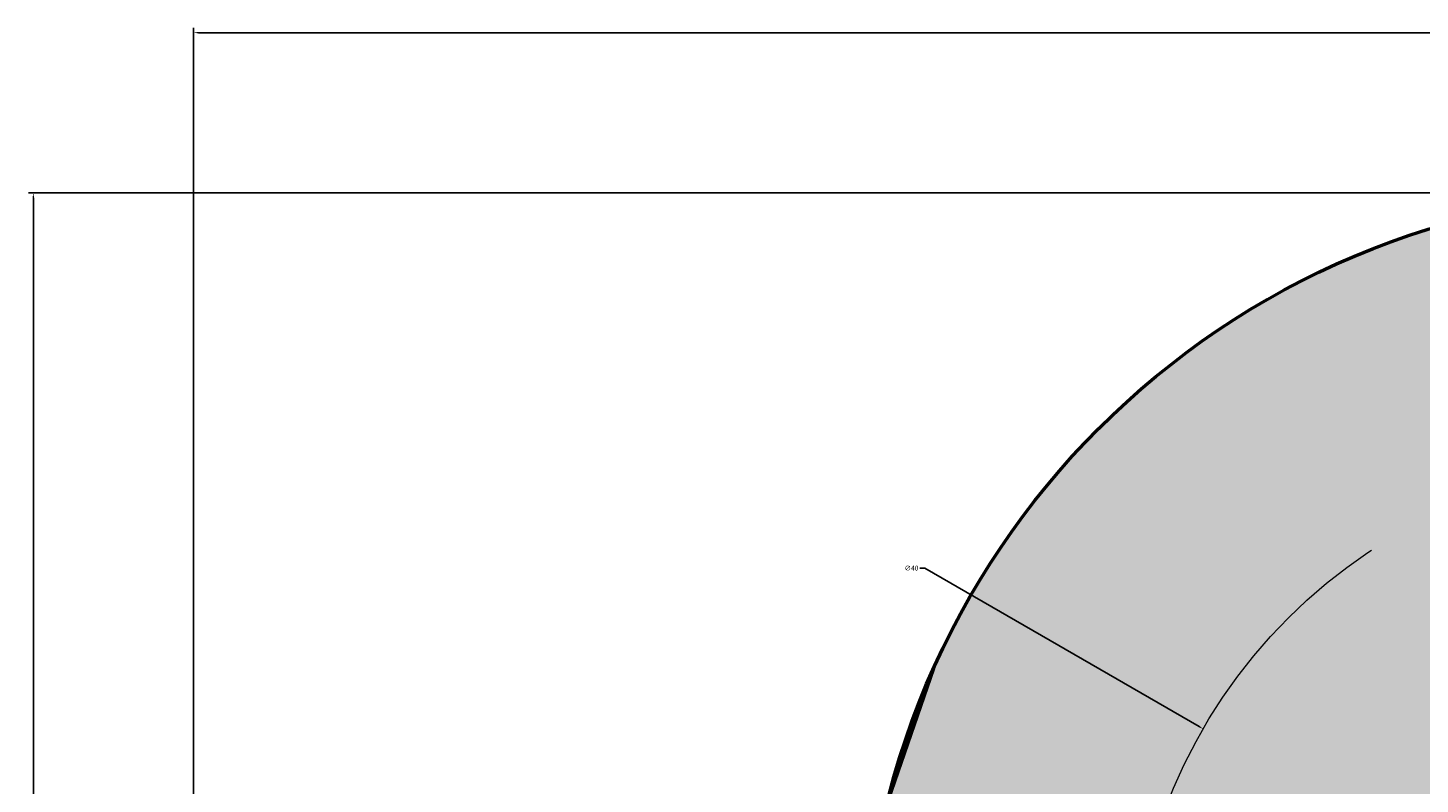
# Model space of a CAD drawing. Units: inches. Extents: x 114 to 236, y -51 to 115.
# Tile 8 of 14: x 114 to 166, y 87 to 115. Entities that reach past the tile are written whole.
import ezdxf

# ---------------------------------------------------------------- set-up
doc = ezdxf.new("R2010")
doc.units = ezdxf.units.IN
doc.header["$MEASUREMENT"] = 0
doc.linetypes.add('CENTER', pattern=[50.8, 31.75, -6.35, 6.35, -6.35])
for name, color, linetype, lineweight in [('M-CNTR', 7, 'CENTER', 18), ('M-DIMS', 2, 'Continuous', 18), ('M-OUTL', 7, 'Continuous', 50)]:
    doc.layers.add(name, color=color, linetype=linetype, lineweight=lineweight)
doc.layers.add('M-HATC', color=7, linetype='Continuous', lineweight=18, true_color=0xffffff)
doc.styles.get("Standard").update_dxf_attribs({"font": 'arial.ttf'})
doc.dimstyles.get("Standard").update_dxf_attribs({"dimtxt": 0.18, "dimasz": 0.18, "dimexe": 0.18, "dimexo": 0.0625, "dimgap": 0.09, "dimtad": 0, "dimtih": 1, "dimtoh": 1, "dimdec": 4, "dimzin": 0, "dimdsep": 46, "dimtxsty": 'Standard', "dimcen": 0.09, "dimadec": 0, "dimazin": 0, "dimtfac": 1, "dimtdec": 4, "dimtofl": 0, "dimtmove": 0, "dimatfit": 3, "dimfxl": 1, "dimtolj": 1, "dimtzin": 0, "dimarcsym": 0})

# ---------------------------------------------------------------- blocks, each defined once
blk = doc.blocks.new('*D3')
at = {"layer": 'Defpoints', "color": 0, "transparency": 16777216}
for p in [(230.229, 115.287), (120.229, 9.307), (230.229, 9.307)]:
    blk.add_point(p, dxfattribs=at)
at = {"layer": 'M-DIMS', "color": 0, "lineweight": -2, "transparency": 16777216}
for p, q in [((120.229, 9.37), (120.229, 115.467)), ((230.229, 9.37), (230.229, 115.467)), ((120.409, 115.287), (174.949, 115.287)), ((230.049, 115.287), (175.509, 115.287))]:
    blk.add_line(p, q, dxfattribs=at)
at = {"layer": 'M-DIMS', "color": 0, "transparency": 16777216}
for points in [[(120.409, 115.317), (120.409, 115.257), (120.229, 115.287)], [(230.049, 115.317), (230.049, 115.257), (230.229, 115.287)]]:
    blk.add_solid(points, dxfattribs=at)
at = {"layer": 'M-DIMS', "color": 0, "transparency": 16777216, "insert": (175.229, 115.287), "char_height": 0.18, "attachment_point": 5}
blk.add_mtext('\\A1;110', dxfattribs=at)
blk = doc.blocks.new('*D4')
at = {"layer": 'Defpoints', "color": 0, "transparency": 16777216}
for p in [(114.249, 109.307), (175.229, 109.307), (135.229, -5.693)]:
    blk.add_point(p, dxfattribs=at)
at = {"layer": 'M-DIMS', "color": 0, "lineweight": -2, "transparency": 16777216}
for p, q in [((175.166, 109.307), (114.069, 109.307)), ((114.249, 109.127), (114.249, 51.989)), ((114.249, -5.513), (114.249, 51.625)), ((135.166, -5.693), (114.069, -5.693))]:
    blk.add_line(p, q, dxfattribs=at)
at = {"layer": 'M-DIMS', "color": 0, "transparency": 16777216}
for points in [[(114.219, 109.127), (114.279, 109.127), (114.249, 109.307)], [(114.219, -5.513), (114.279, -5.513), (114.249, -5.693)]]:
    blk.add_solid(points, dxfattribs=at)
at = {"layer": 'M-DIMS', "color": 0, "transparency": 16777216, "insert": (114.249, 51.807), "char_height": 0.18, "attachment_point": 5}
blk.add_mtext('\\A1;115', dxfattribs=at)
blk = doc.blocks.new('*D8')
at = {"layer": 'Defpoints', "color": 0, "transparency": 16777216}
for p in [(197.149, 99.789), (153.308, 58.825)]:
    blk.add_point(p, dxfattribs=at)
at = {"layer": 'M-DIMS', "color": 0, "lineweight": -2, "transparency": 16777216}
for p, q in [((210.301, 112.078), (197.28, 99.912)), ((210.481, 112.078), (210.301, 112.078)), ((175.139, 79.307), (175.319, 79.307)), ((175.229, 79.217), (175.229, 79.397))]:
    blk.add_line(p, q, dxfattribs=at)
at = {"layer": 'M-DIMS', "color": 0, "transparency": 16777216}
blk.add_solid([(197.26, 99.934), (197.301, 99.89), (197.149, 99.789)], dxfattribs=at)
at = {"layer": 'M-DIMS', "color": 0, "transparency": 16777216, "insert": (210.797, 112.078), "char_height": 0.18, "attachment_point": 5}
blk.add_mtext('\\A1;∅60', dxfattribs=at)
blk = doc.blocks.new('*D9')
at = {"layer": 'Defpoints', "color": 0, "transparency": 16777216}
for p in [(157.908, 89.307), (192.549, 69.307)]:
    blk.add_point(p, dxfattribs=at)
at = {"layer": 'M-DIMS', "color": 0, "lineweight": -2, "transparency": 16777216}
for p, q in [((147.336, 95.307), (147.516, 95.307)), ((147.516, 95.307), (157.752, 89.397)), ((175.139, 79.307), (175.319, 79.307)), ((175.229, 79.217), (175.229, 79.397))]:
    blk.add_line(p, q, dxfattribs=at)
at = {"layer": 'M-DIMS', "color": 0, "transparency": 16777216}
blk.add_solid([(157.767, 89.423), (157.737, 89.371), (157.908, 89.307)], dxfattribs=at)
at = {"layer": 'M-DIMS', "color": 0, "transparency": 16777216, "insert": (147.019, 95.307), "char_height": 0.18, "attachment_point": 5}
blk.add_mtext('\\A1;∅40', dxfattribs=at)

msp = doc.modelspace()

# ---------------------------------------------------------------- hatches: boundary and pattern name
at = {"layer": 'M-HATC'}
h = msp.add_hatch(color=256, dxfattribs=at)
h.set_gradient(color1=(19, 155, 72), color2=(255, 255, 0), tint=1, name='HEMISPHERICAL')
h.paths.add_polyline_path([(147.853, 91.577), (146.105, 86.505, 0.060651), (145.229, 79.307, 1), (205.229, 79.307, 0.060651), (204.352, 86.505), (202.605, 91.577, 0.647643)])
h.paths.add_polyline_path([(180.229, 99.307, -0.031342), (180.189, 98.682, -0.27393), (194.604, 84.268, -0.451416), (200.229, 79.307, -0.451416), (194.604, 74.346, -0.27393), (180.189, 59.932, -0.031342), (180.229, 59.307, -1), (170.229, 59.307, -0.031342), (170.268, 59.932, -0.27393), (155.854, 74.346, -0.451416), (150.229, 79.307, -0.451416), (155.854, 84.268, -0.27393), (170.268, 98.682, -0.031342), (170.229, 99.307, -1)], flags=16)
h.paths.add_polyline_path([(183.229, 79.307, -1), (167.229, 79.307, -1)], flags=0)
h.paths.add_polyline_path([(155.854, 84.268, -0.377964), (160.229, 79.307, -0.377964), (155.854, 74.346, 0.27393), (170.268, 59.932, -0.881917), (180.189, 59.932, 0.27393), (194.604, 74.346, -0.377964), (190.229, 79.307, -0.377964), (194.604, 84.268, 0.27393), (180.189, 98.682, -0.881917), (170.268, 98.682, 0.27393)], flags=0)

# ---------------------------------------------------------------- linework, layer by layer
at = {"layer": 'M-CNTR'}
msp.add_circle((175.229, 79.307), 20, dxfattribs=at)
at = {"layer": 'M-OUTL'}
msp.add_line((120.523, 12.263), (147.853, 91.577), dxfattribs=at)
msp.add_circle((175.229, 79.307), 30, dxfattribs=at)

# ---------------------------------------------------------------- dimensions: what is measured, and where the dimension line sits
at = {"layer": 'M-DIMS'}
dim = msp.add_linear_dim(base=(230.229, 115.287), p1=(120.229, 9.307), p2=(230.229, 9.307), dimstyle='Standard', override={"dimdec": 0, "dimlfac": 1, "dimrnd": 0, "dimzin": 0, "dimdsep": 46, "dimlunit": 2}, dxfattribs=at)
dim.commit()
dim.dimension.update_dxf_attribs({"geometry": '*D3', "text_midpoint": (175.229, 115.287)})
for p1, p2, picture, middle in [((153.308, 58.825), (197.149, 99.789), '*D8', (210.797, 112.078)), ((192.549, 69.307), (157.908, 89.307), '*D9', (147.019, 95.307))]:
    dim = msp.add_diameter_dim_2p(p1=p1, p2=p2, dimstyle='Standard', override={"dimdec": 0, "dimlfac": 1, "dimrnd": 0, "dimzin": 0, "dimdsep": 46, "dimlunit": 2}, dxfattribs=at)
    dim.commit()
    dim.dimension.update_dxf_attribs({"geometry": picture, "text_midpoint": middle, "dimtype": 163})
dim = msp.add_linear_dim(base=(114.249, 109.307), p1=(135.229, -5.693), p2=(175.229, 109.307), angle=90, dimstyle='Standard', override={"dimdec": 0, "dimlfac": 1, "dimrnd": 0, "dimzin": 0, "dimdsep": 46, "dimlunit": 2}, dxfattribs=at)
dim.commit()
dim.dimension.update_dxf_attribs({"geometry": '*D4', "text_midpoint": (114.249, 51.807)})

doc.saveas('drawing.dxf')
